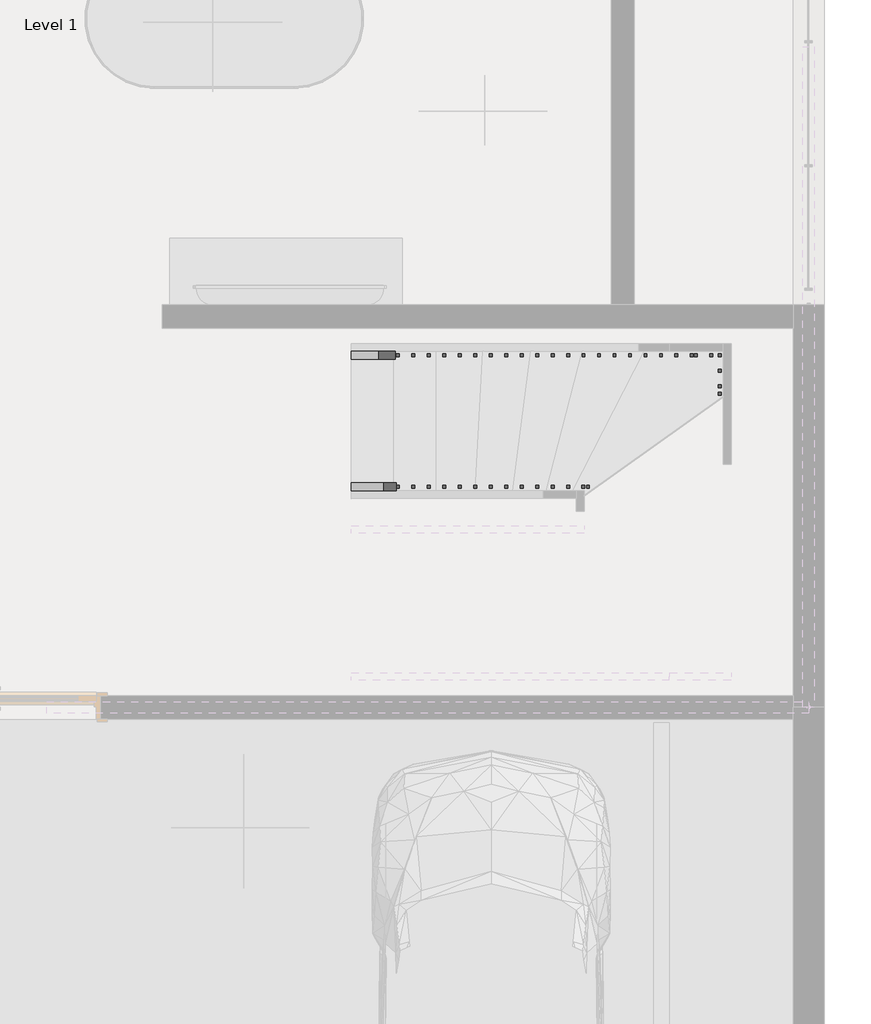
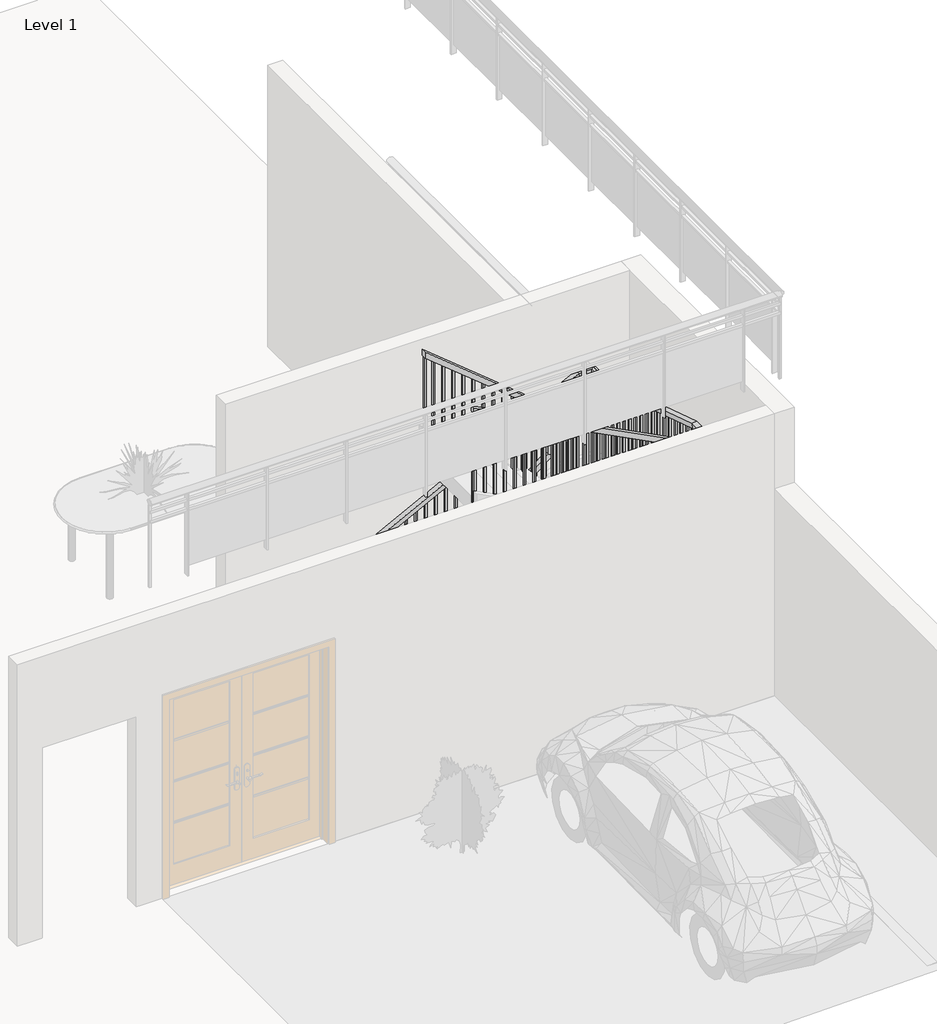
# One storey, part 4 of 6: 2 railings.
"""IFC4 building model written with IfcOpenShell, lengths in millimetres."""

from ifc_helpers import new_model, si_unit, frame, origin, place, context, project, spatial, polyline, outline, extrude, faceted_brep, element, save

model = new_model("IFC4")

# Units and contexts
model_context = context("Model", 3, world=origin())
ifc_project = project(units=[si_unit("LENGTHUNIT", "METRE", prefix="MILLI")], contexts=[model_context])

# Site, building, storey
site = spatial("IfcSite", under=ifc_project)
building = spatial("IfcBuilding", under=site)
storey = spatial("IfcBuildingStorey", under=building, Name="Level 1", Elevation=0.0)

# Railings
placement = place(None, origin())
element("IfcRailing", 1, ObjectType="Handrail - Rectangular", at=placement, inside=storey, context=model_context, shape_type="SolidModel", body=[
    faceted_brep([(-5314.5158104, 2829.6271763, 1025.2529681), (-5314.5158104, 2829.6271763, 959.7067088), (-5314.5158104, 2778.8271763, 959.7067088), (-5314.5158104, 2778.8271763, 1025.2529681), (-3862.9841185, 2829.6271763, 2208.7848338), (-3812.1841185, 2829.6271763, 2184.659247), (-3812.1841185, 2778.8271763, 2184.659247), (-3862.9841185, 2778.8271763, 2208.7848338), (-3862.9841185, 2829.6271763, 2414.6281882), (-3812.1841185, 2829.6271763, 2363.8281882), (-3812.1841185, 2778.8271763, 2363.8281882), (-3862.9841185, 2778.8271763, 2414.6281882), (-3735.9841185, 2829.6271763, 2414.6281882), (-3735.9841185, 2829.6271763, 2363.8281882), (-3786.7841185, 2778.8271763, 2363.8281882), (-3786.7841185, 2778.8271763, 2414.6281882), (-3735.9841185, 2702.6271763, 2414.6281882), (-3735.9841185, 2673.5058424, 2363.8281882), (-3786.7841185, 2673.5058424, 2363.8281882), (-3786.7841185, 2702.6271763, 2414.6281882), (-3735.9841185, 2575.6271763, 2631.5051451), (-3735.9841185, 2524.8271763, 2617.7256424), (-3786.7841185, 2524.8271763, 2617.7256424), (-3786.7841185, 2575.6271763, 2631.5051451), (-3735.9841185, 2575.6271763, 2837.3484995), (-3735.9841185, 2524.8271763, 2786.5484995), (-3786.7841185, 2524.8271763, 2786.5484995), (-3786.7841185, 2575.6271763, 2837.3484995), (-3735.9841185, 2448.6271763, 2837.3484995), (-3735.9841185, 2448.6271763, 2786.5484995), (-3786.7841185, 2499.4271763, 2786.5484995), (-3786.7841185, 2499.4271763, 2837.3484995), (-3862.9841185, 2448.6271763, 2837.3484995), (-3881.0695316, 2448.6271763, 2786.5484995), (-3881.0695316, 2499.4271763, 2786.5484995), (-3862.9841185, 2499.4271763, 2837.3484995), (-5314.5158104, 2448.6271763, 4020.8803652), (-5314.5158104, 2499.4271763, 4020.8803652), (-5314.5158104, 2499.4271763, 3955.3341059), (-5314.5158104, 2448.6271763, 3955.3341059)], [[[0, 1, 2, 3]], [[1, 0, 4, 5]], [[2, 1, 5, 6]], [[3, 2, 6, 7]], [[0, 3, 7, 4]], [[5, 4, 8, 9]], [[6, 5, 9, 10]], [[7, 6, 10, 11]], [[4, 7, 11, 8]], [[9, 8, 12, 13]], [[10, 9, 13, 14]], [[11, 10, 14, 15]], [[8, 11, 15, 12]], [[13, 12, 16, 17]], [[14, 13, 17, 18]], [[15, 14, 18, 19]], [[12, 15, 19, 16]], [[17, 16, 20, 21]], [[18, 17, 21, 22]], [[19, 18, 22, 23]], [[16, 19, 23, 20]], [[21, 20, 24, 25]], [[22, 21, 25, 26]], [[23, 22, 26, 27]], [[20, 23, 27, 24]], [[25, 24, 28, 29]], [[26, 25, 29, 30]], [[27, 26, 30, 31]], [[24, 27, 31, 28]], [[29, 28, 32, 33]], [[30, 29, 33, 34]], [[31, 30, 34, 35]], [[28, 31, 35, 32]], [[36, 37, 38, 39]], [[33, 32, 36, 39]], [[34, 33, 39, 38]], [[35, 34, 38, 37]], [[32, 35, 37, 36]]]),
    extrude(outline(polyline([(3866.2231262, -5205.2264749), (3881.7558784, -5224.2764749), (2878.6666667, -5224.2764749), (2878.6666667, -5205.2264749), (3866.2231262, -5205.2264749)])), frame((0.0, 2464.5021763, 0.0), z_axis=(0.0, 1.0, 0.0), x_axis=(0.0, 0.0, 1.0)), (0.0, 0.0, 1.0), 19.05),
    extrude(outline(polyline([(3783.3817813, -5103.6264749), (3798.9145334, -5122.6764749), (2878.6666667, -5122.6764749), (2878.6666667, -5103.6264749), (3783.3817813, -5103.6264749)])), frame((0.0, 2464.5021763, 0.0), z_axis=(0.0, 1.0, 0.0), x_axis=(0.0, 0.0, 1.0)), (0.0, 0.0, 1.0), 19.05),
    extrude(outline(polyline([(3700.5404364, -5002.0264749), (3716.0731885, -5021.0764749), (2709.3333333, -5021.0764749), (2709.3333333, -5002.0264749), (3700.5404364, -5002.0264749)])), frame((0.0, 2464.5021763, 0.0), z_axis=(0.0, 1.0, 0.0), x_axis=(0.0, 0.0, 1.0)), (0.0, 0.0, 1.0), 19.05),
    extrude(outline(polyline([(3617.6990914, -4900.4264749), (3633.2318436, -4919.4764749), (2709.3333333, -4919.4764749), (2709.3333333, -4900.4264749), (3617.6990914, -4900.4264749)])), frame((0.0, 2464.5021763, 0.0), z_axis=(0.0, 1.0, 0.0), x_axis=(0.0, 0.0, 1.0)), (0.0, 0.0, 1.0), 19.05),
    extrude(outline(polyline([(3534.8577465, -4798.8264749), (3550.3904987, -4817.8764749), (2709.3333333, -4817.8764749), (2709.3333333, -4798.8264749), (3534.8577465, -4798.8264749)])), frame((0.0, 2464.5021763, 0.0), z_axis=(0.0, 1.0, 0.0), x_axis=(0.0, 0.0, 1.0)), (0.0, 0.0, 1.0), 19.05),
    extrude(outline(polyline([(3452.0164016, -4697.2264749), (3467.5491538, -4716.2764749), (2540.0, -4716.2764749), (2540.0, -4697.2264749), (3452.0164016, -4697.2264749)])), frame((0.0, 2464.5021763, 0.0), z_axis=(0.0, 1.0, 0.0), x_axis=(0.0, 0.0, 1.0)), (0.0, 0.0, 1.0), 19.05),
    extrude(outline(polyline([(3369.1750567, -4595.6264749), (3384.7078088, -4614.6764749), (2540.0, -4614.6764749), (2540.0, -4595.6264749), (3369.1750567, -4595.6264749)])), frame((0.0, 2464.5021763, 0.0), z_axis=(0.0, 1.0, 0.0), x_axis=(0.0, 0.0, 1.0)), (0.0, 0.0, 1.0), 19.05),
    extrude(outline(polyline([(3286.3337117, -4494.0264749), (3301.8664639, -4513.0764749), (2540.0, -4513.0764749), (2540.0, -4494.0264749), (3286.3337117, -4494.0264749)])), frame((0.0, 2464.5021763, 0.0), z_axis=(0.0, 1.0, 0.0), x_axis=(0.0, 0.0, 1.0)), (0.0, 0.0, 1.0), 19.05),
    extrude(outline(polyline([(3203.4923668, -4392.4264749), (3219.025119, -4411.4764749), (2370.6666667, -4411.4764749), (2370.6666667, -4392.4264749), (3203.4923668, -4392.4264749)])), frame((0.0, 2464.5021763, 0.0), z_axis=(0.0, 1.0, 0.0), x_axis=(0.0, 0.0, 1.0)), (0.0, 0.0, 1.0), 19.05),
    extrude(outline(polyline([(3120.6510219, -4290.8264749), (3136.1837741, -4309.8764749), (2370.6666667, -4309.8764749), (2370.6666667, -4290.8264749), (3120.6510219, -4290.8264749)])), frame((0.0, 2464.5021763, 0.0), z_axis=(0.0, 1.0, 0.0), x_axis=(0.0, 0.0, 1.0)), (0.0, 0.0, 1.0), 19.05),
    extrude(outline(polyline([(3037.809677, -4189.2264749), (3053.3424291, -4208.2764749), (2201.3333333, -4208.2764749), (2201.3333333, -4189.2264749), (3037.809677, -4189.2264749)])), frame((0.0, 2464.5021763, 0.0), z_axis=(0.0, 1.0, 0.0), x_axis=(0.0, 0.0, 1.0)), (0.0, 0.0, 1.0), 19.05),
    extrude(outline(polyline([(2954.9683321, -4087.6264749), (2970.5010842, -4106.6764749), (2201.3333333, -4106.6764749), (2201.3333333, -4087.6264749), (2954.9683321, -4087.6264749)])), frame((0.0, 2464.5021763, 0.0), z_axis=(0.0, 1.0, 0.0), x_axis=(0.0, 0.0, 1.0)), (0.0, 0.0, 1.0), 19.05),
    extrude(outline(polyline([(2872.1269871, -3986.0264749), (2887.6597393, -4005.0764749), (2032.0, -4005.0764749), (2032.0, -3986.0264749), (2872.1269871, -3986.0264749)])), frame((0.0, 2464.5021763, 0.0), z_axis=(0.0, 1.0, 0.0), x_axis=(0.0, 0.0, 1.0)), (0.0, 0.0, 1.0), 19.05),
    extrude(outline(polyline([(2789.2856422, -3884.4264749), (2804.8183944, -3903.4764749), (2032.0, -3903.4764749), (2032.0, -3884.4264749), (2789.2856422, -3884.4264749)])), frame((0.0, 2464.5021763, 0.0), z_axis=(0.0, 1.0, 0.0), x_axis=(0.0, 0.0, 1.0)), (0.0, 0.0, 1.0), 19.05),
    extrude(outline(polyline([(2576.7162725, 2529.115018), (2595.7662725, 2496.5834745), (2595.7662725, 1524.0), (2576.7162725, 1524.0), (2576.7162725, 2529.115018)])), frame((-3770.9091185, 0.0, 0.0), z_axis=(1.0, 0.0, 0.0), x_axis=(0.0, 1.0, 0.0)), (0.0, 0.0, 1.0), 19.05),
    extrude(outline(polyline([(2678.3162725, 2355.6134525), (2697.3662725, 2323.0819089), (2697.3662725, 1524.0), (2678.3162725, 1524.0), (2678.3162725, 2355.6134525)])), frame((-3770.9091185, 0.0, 0.0), z_axis=(1.0, 0.0, 0.0), x_axis=(0.0, 1.0, 0.0)), (0.0, 0.0, 1.0), 19.05),
    extrude(outline(polyline([(2127.2519138, -3882.5908104), (2111.7191617, -3901.6408104), (1016.0, -3901.6408104), (1016.0, -3882.5908104), (2127.2519138, -3882.5908104)])), frame((0.0, 2794.7021763, 0.0), z_axis=(0.0, 1.0, 0.0), x_axis=(0.0, 0.0, 1.0)), (0.0, 0.0, 1.0), 19.05),
    extrude(outline(polyline([(2044.4105689, -3984.1908104), (2028.8778167, -4003.2408104), (1016.0, -4003.2408104), (1016.0, -3984.1908104), (2044.4105689, -3984.1908104)])), frame((0.0, 2794.7021763, 0.0), z_axis=(0.0, 1.0, 0.0), x_axis=(0.0, 0.0, 1.0)), (0.0, 0.0, 1.0), 19.05),
    extrude(outline(polyline([(1961.569224, -4085.7908104), (1946.0364718, -4104.8408104), (846.6666667, -4104.8408104), (846.6666667, -4085.7908104), (1961.569224, -4085.7908104)])), frame((0.0, 2794.7021763, 0.0), z_axis=(0.0, 1.0, 0.0), x_axis=(0.0, 0.0, 1.0)), (0.0, 0.0, 1.0), 19.05),
    extrude(outline(polyline([(1878.7278791, -4187.3908104), (1863.1951269, -4206.4408104), (846.6666667, -4206.4408104), (846.6666667, -4187.3908104), (1878.7278791, -4187.3908104)])), frame((0.0, 2794.7021763, 0.0), z_axis=(0.0, 1.0, 0.0), x_axis=(0.0, 0.0, 1.0)), (0.0, 0.0, 1.0), 19.05),
    extrude(outline(polyline([(1795.8865341, -4288.9908104), (1780.353782, -4308.0408104), (677.3333333, -4308.0408104), (677.3333333, -4288.9908104), (1795.8865341, -4288.9908104)])), frame((0.0, 2794.7021763, 0.0), z_axis=(0.0, 1.0, 0.0), x_axis=(0.0, 0.0, 1.0)), (0.0, 0.0, 1.0), 19.05),
    extrude(outline(polyline([(1713.0451892, -4390.5908104), (1697.5124371, -4409.6408104), (677.3333333, -4409.6408104), (677.3333333, -4390.5908104), (1713.0451892, -4390.5908104)])), frame((0.0, 2794.7021763, 0.0), z_axis=(0.0, 1.0, 0.0), x_axis=(0.0, 0.0, 1.0)), (0.0, 0.0, 1.0), 19.05),
    extrude(outline(polyline([(1630.2038443, -4492.1908104), (1614.6710921, -4511.2408104), (508.0, -4511.2408104), (508.0, -4492.1908104), (1630.2038443, -4492.1908104)])), frame((0.0, 2794.7021763, 0.0), z_axis=(0.0, 1.0, 0.0), x_axis=(0.0, 0.0, 1.0)), (0.0, 0.0, 1.0), 19.05),
    extrude(outline(polyline([(1547.3624994, -4593.7908104), (1531.8297472, -4612.8408104), (508.0, -4612.8408104), (508.0, -4593.7908104), (1547.3624994, -4593.7908104)])), frame((0.0, 2794.7021763, 0.0), z_axis=(0.0, 1.0, 0.0), x_axis=(0.0, 0.0, 1.0)), (0.0, 0.0, 1.0), 19.05),
    extrude(outline(polyline([(1464.5211545, -4695.3908104), (1448.9884023, -4714.4408104), (508.0, -4714.4408104), (508.0, -4695.3908104), (1464.5211545, -4695.3908104)])), frame((0.0, 2794.7021763, 0.0), z_axis=(0.0, 1.0, 0.0), x_axis=(0.0, 0.0, 1.0)), (0.0, 0.0, 1.0), 19.05),
    extrude(outline(polyline([(1381.6798095, -4796.9908104), (1366.1470574, -4816.0408104), (338.6666667, -4816.0408104), (338.6666667, -4796.9908104), (1381.6798095, -4796.9908104)])), frame((0.0, 2794.7021763, 0.0), z_axis=(0.0, 1.0, 0.0), x_axis=(0.0, 0.0, 1.0)), (0.0, 0.0, 1.0), 19.05),
    extrude(outline(polyline([(1298.8384646, -4898.5908104), (1283.3057124, -4917.6408104), (338.6666667, -4917.6408104), (338.6666667, -4898.5908104), (1298.8384646, -4898.5908104)])), frame((0.0, 2794.7021763, 0.0), z_axis=(0.0, 1.0, 0.0), x_axis=(0.0, 0.0, 1.0)), (0.0, 0.0, 1.0), 19.05),
    extrude(outline(polyline([(1215.9971197, -5000.1908104), (1200.4643675, -5019.2408104), (338.6666667, -5019.2408104), (338.6666667, -5000.1908104), (1215.9971197, -5000.1908104)])), frame((0.0, 2794.7021763, 0.0), z_axis=(0.0, 1.0, 0.0), x_axis=(0.0, 0.0, 1.0)), (0.0, 0.0, 1.0), 19.05),
    extrude(outline(polyline([(1133.1557748, -5101.7908104), (1117.6230226, -5120.8408104), (169.3333333, -5120.8408104), (169.3333333, -5101.7908104), (1133.1557748, -5101.7908104)])), frame((0.0, 2794.7021763, 0.0), z_axis=(0.0, 1.0, 0.0), x_axis=(0.0, 0.0, 1.0)), (0.0, 0.0, 1.0), 19.05),
    extrude(outline(polyline([(1050.3144298, -5203.3908104), (1034.7816777, -5222.4408104), (169.3333333, -5222.4408104), (169.3333333, -5203.3908104), (1050.3144298, -5203.3908104)])), frame((0.0, 2794.7021763, 0.0), z_axis=(0.0, 1.0, 0.0), x_axis=(0.0, 0.0, 1.0)), (0.0, 0.0, 1.0), 19.05),
    extrude(outline(polyline([(-3782.8264749, 2483.5521763), (-3782.8264749, 2464.5021763), (-3801.8764749, 2464.5021763), (-3801.8764749, 2483.5521763), (-3782.8264749, 2483.5521763)])), frame((0.0, 0.0, 1862.6666667), z_axis=(0.0, 0.0, 1.0), x_axis=(1.0, 0.0, 0.0)), (0.0, 0.0, 1.0), 923.8818329),
    extrude(outline(polyline([(-3770.9091185, 2483.5521763), (-3751.8591185, 2483.5521763), (-3751.8591185, 2464.5021763), (-3770.9091185, 2464.5021763), (-3770.9091185, 2483.5521763)])), frame((0.0, 0.0, 1862.6666667), z_axis=(0.0, 0.0, 1.0), x_axis=(1.0, 0.0, 0.0)), (0.0, 0.0, 1.0), 923.8818329),
    extrude(outline(polyline([(-3770.9091185, 2498.33808), (-3751.8591185, 2498.33808), (-3751.8591185, 2479.28808), (-3770.9091185, 2479.28808), (-3770.9091185, 2498.33808)])), frame((0.0, 0.0, 1693.3333333), z_axis=(0.0, 0.0, 1.0), x_axis=(1.0, 0.0, 0.0)), (0.0, 0.0, 1.0), 1093.2151662),
    extrude(outline(polyline([(-3770.9091185, 2798.9662725), (-3751.8591185, 2798.9662725), (-3751.8591185, 2779.9162725), (-3770.9091185, 2779.9162725), (-3770.9091185, 2798.9662725)])), frame((0.0, 0.0, 1354.6666667), z_axis=(0.0, 0.0, 1.0), x_axis=(1.0, 0.0, 0.0)), (0.0, 0.0, 1.0), 1009.1615215),
    extrude(outline(polyline([(-3770.9091185, 2794.7021763), (-3770.9091185, 2813.7521763), (-3751.8591185, 2813.7521763), (-3751.8591185, 2794.7021763), (-3770.9091185, 2794.7021763)])), frame((0.0, 0.0, 1185.3333333), z_axis=(0.0, 0.0, 1.0), x_axis=(1.0, 0.0, 0.0)), (0.0, 0.0, 1.0), 1178.4948549),
    extrude(outline(polyline([(-3801.8764749, 2794.7021763), (-3801.8764749, 2813.7521763), (-3782.8264749, 2813.7521763), (-3782.8264749, 2794.7021763), (-3801.8764749, 2794.7021763)])), frame((0.0, 0.0, 1185.3333333), z_axis=(0.0, 0.0, 1.0), x_axis=(1.0, 0.0, 0.0)), (0.0, 0.0, 1.0), 1178.4948549),
    extrude(outline(polyline([(3939.8013537, -5295.4658104), (3955.3341059, -5314.5158104), (2878.6666667, -5314.5158104), (2878.6666667, -5295.4658104), (3939.8013537, -5295.4658104)])), frame((0.0, 2464.5021763, 0.0), z_axis=(0.0, 1.0, 0.0), x_axis=(0.0, 0.0, 1.0)), (0.0, 0.0, 1.0), 19.05),
    extrude(outline(polyline([(975.239461, -5295.4658104), (959.7067088, -5314.5158104), (169.3333333, -5314.5158104), (169.3333333, -5295.4658104), (975.239461, -5295.4658104)])), frame((0.0, 2794.7021763, 0.0), z_axis=(0.0, 1.0, 0.0), x_axis=(0.0, 0.0, 1.0)), (0.0, 0.0, 1.0), 19.05),
])
element("IfcRailing", 2, ObjectType="Handrail - Rectangular", at=placement, inside=storey, context=model_context, shape_type="SolidModel", body=[
    faceted_brep([(-5314.5158104, 3693.2271763, 1109.0771751), (-5314.5158104, 3693.2271763, 1051.9280057), (-5314.5158104, 3642.4271763, 1051.9280057), (-5314.5158104, 3642.4271763, 1109.0771751), (-3054.5339539, 3693.2271763, 2273.7644996), (-3042.2139026, 3693.2271763, 2222.9644996), (-3042.2139026, 3642.4271763, 2222.9644996), (-3054.5339539, 3642.4271763, 2273.7644996), (-2872.3841185, 3693.2271763, 2273.7644996), (-2872.3841185, 3693.2271763, 2222.9644996), (-2923.1841185, 3642.4271763, 2222.9644996), (-2923.1841185, 3642.4271763, 2273.7644996), (-2872.3841185, 3416.0732236, 2273.7644996), (-2872.3841185, 3408.1226475, 2222.9644996), (-2923.1841185, 3408.1226475, 2222.9644996), (-2923.1841185, 3416.0732236, 2273.7644996), (-2872.3841185, 1862.1811289, 2772.3688337), (-2872.3841185, 1854.2305527, 2721.5688337), (-2923.1841185, 1854.2305527, 2721.5688337), (-2923.1841185, 1862.1811289, 2772.3688337), (-2872.3841185, 1585.0271763, 2772.3688337), (-2872.3841185, 1585.0271763, 2721.5688337), (-2923.1841185, 1635.8271763, 2721.5688337), (-2923.1841185, 1635.8271763, 2772.3688337), (-3054.5339539, 1585.0271763, 2772.3688337), (-3066.8540052, 1585.0271763, 2721.5688337), (-3066.8540052, 1635.8271763, 2721.5688337), (-3054.5339539, 1635.8271763, 2772.3688337), (-5314.5158104, 1585.0271763, 3937.0561582), (-5314.5158104, 1635.8271763, 3937.0561582), (-5314.5158104, 1635.8271763, 3879.9069889), (-5314.5158104, 1585.0271763, 3879.9069889)], [[[0, 1, 2, 3]], [[1, 0, 4, 5]], [[2, 1, 5, 6]], [[3, 2, 6, 7]], [[0, 3, 7, 4]], [[5, 4, 8, 9]], [[6, 5, 9, 10]], [[7, 6, 10, 11]], [[4, 7, 11, 8]], [[9, 8, 12, 13]], [[10, 9, 13, 14]], [[11, 10, 14, 15]], [[8, 11, 15, 12]], [[13, 12, 16, 17]], [[14, 13, 17, 18]], [[15, 14, 18, 19]], [[12, 15, 19, 16]], [[17, 16, 20, 21]], [[18, 17, 21, 22]], [[19, 18, 22, 23]], [[16, 19, 23, 20]], [[21, 20, 24, 25]], [[22, 21, 25, 26]], [[23, 22, 26, 27]], [[20, 23, 27, 24]], [[28, 29, 30, 31]], [[25, 24, 28, 31]], [[26, 25, 31, 30]], [[27, 26, 30, 29]], [[24, 27, 29, 28]]]),
    extrude(outline(polyline([(3872.0443296, -5299.2589539), (2878.6666667, -5299.2589539), (2878.6666667, -5280.2089539), (3862.2268642, -5280.2089539), (3872.0443296, -5299.2589539)])), frame((0.0, 1600.9021763, 0.0), z_axis=(0.0, 1.0, 0.0), x_axis=(0.0, 0.0, 1.0)), (0.0, 0.0, 1.0), 19.05),
    extrude(outline(polyline([(3819.6845145, -5197.6589539), (2878.6666667, -5197.6589539), (2878.6666667, -5178.6089539), (3809.8670491, -5178.6089539), (3819.6845145, -5197.6589539)])), frame((0.0, 1600.9021763, 0.0), z_axis=(0.0, 1.0, 0.0), x_axis=(0.0, 0.0, 1.0)), (0.0, 0.0, 1.0), 19.05),
    extrude(outline(polyline([(3767.3246993, -5096.0589539), (2878.6666667, -5096.0589539), (2878.6666667, -5077.0089539), (3757.507234, -5077.0089539), (3767.3246993, -5096.0589539)])), frame((0.0, 1600.9021763, 0.0), z_axis=(0.0, 1.0, 0.0), x_axis=(0.0, 0.0, 1.0)), (0.0, 0.0, 1.0), 19.05),
    extrude(outline(polyline([(3714.9648842, -4994.4589539), (2709.3333333, -4994.4589539), (2709.3333333, -4975.4089539), (3705.1474189, -4975.4089539), (3714.9648842, -4994.4589539)])), frame((0.0, 1600.9021763, 0.0), z_axis=(0.0, 1.0, 0.0), x_axis=(0.0, 0.0, 1.0)), (0.0, 0.0, 1.0), 19.05),
    extrude(outline(polyline([(3662.6050691, -4892.8589539), (2709.3333333, -4892.8589539), (2709.3333333, -4873.8089539), (3652.7876038, -4873.8089539), (3662.6050691, -4892.8589539)])), frame((0.0, 1600.9021763, 0.0), z_axis=(0.0, 1.0, 0.0), x_axis=(0.0, 0.0, 1.0)), (0.0, 0.0, 1.0), 19.05),
    extrude(outline(polyline([(3610.245254, -4791.2589539), (2709.3333333, -4791.2589539), (2709.3333333, -4772.2089539), (3600.4277887, -4772.2089539), (3610.245254, -4791.2589539)])), frame((0.0, 1600.9021763, 0.0), z_axis=(0.0, 1.0, 0.0), x_axis=(0.0, 0.0, 1.0)), (0.0, 0.0, 1.0), 19.05),
    extrude(outline(polyline([(3557.8854389, -4689.6589539), (2540.0, -4689.6589539), (2540.0, -4670.6089539), (3548.0679735, -4670.6089539), (3557.8854389, -4689.6589539)])), frame((0.0, 1600.9021763, 0.0), z_axis=(0.0, 1.0, 0.0), x_axis=(0.0, 0.0, 1.0)), (0.0, 0.0, 1.0), 19.05),
    extrude(outline(polyline([(3505.5256238, -4588.0589539), (2540.0, -4588.0589539), (2540.0, -4569.0089539), (3495.7081584, -4569.0089539), (3505.5256238, -4588.0589539)])), frame((0.0, 1600.9021763, 0.0), z_axis=(0.0, 1.0, 0.0), x_axis=(0.0, 0.0, 1.0)), (0.0, 0.0, 1.0), 19.05),
    extrude(outline(polyline([(3453.1658086, -4486.4589539), (2540.0, -4486.4589539), (2540.0, -4467.4089539), (3443.3483433, -4467.4089539), (3453.1658086, -4486.4589539)])), frame((0.0, 1600.9021763, 0.0), z_axis=(0.0, 1.0, 0.0), x_axis=(0.0, 0.0, 1.0)), (0.0, 0.0, 1.0), 19.05),
    extrude(outline(polyline([(3400.8059935, -4384.8589539), (2370.6666667, -4384.8589539), (2370.6666667, -4365.8089539), (3390.9885282, -4365.8089539), (3400.8059935, -4384.8589539)])), frame((0.0, 1600.9021763, 0.0), z_axis=(0.0, 1.0, 0.0), x_axis=(0.0, 0.0, 1.0)), (0.0, 0.0, 1.0), 19.05),
    extrude(outline(polyline([(3348.4461784, -4283.2589539), (2370.6666667, -4283.2589539), (2370.6666667, -4264.2089539), (3338.6287131, -4264.2089539), (3348.4461784, -4283.2589539)])), frame((0.0, 1600.9021763, 0.0), z_axis=(0.0, 1.0, 0.0), x_axis=(0.0, 0.0, 1.0)), (0.0, 0.0, 1.0), 19.05),
    extrude(outline(polyline([(3296.0863633, -4181.6589539), (2370.6666667, -4181.6589539), (2370.6666667, -4162.6089539), (3286.268898, -4162.6089539), (3296.0863633, -4181.6589539)])), frame((0.0, 1600.9021763, 0.0), z_axis=(0.0, 1.0, 0.0), x_axis=(0.0, 0.0, 1.0)), (0.0, 0.0, 1.0), 19.05),
    extrude(outline(polyline([(3243.7265482, -4080.0589539), (2201.3333333, -4080.0589539), (2201.3333333, -4061.0089539), (3233.9090828, -4061.0089539), (3243.7265482, -4080.0589539)])), frame((0.0, 1600.9021763, 0.0), z_axis=(0.0, 1.0, 0.0), x_axis=(0.0, 0.0, 1.0)), (0.0, 0.0, 1.0), 19.05),
    extrude(outline(polyline([(3191.3667331, -3978.4589539), (2201.3333333, -3978.4589539), (2201.3333333, -3959.4089539), (3181.5492677, -3959.4089539), (3191.3667331, -3978.4589539)])), frame((0.0, 1600.9021763, 0.0), z_axis=(0.0, 1.0, 0.0), x_axis=(0.0, 0.0, 1.0)), (0.0, 0.0, 1.0), 19.05),
    extrude(outline(polyline([(3139.0069179, -3876.8589539), (2201.3333333, -3876.8589539), (2201.3333333, -3857.8089539), (3129.1894526, -3857.8089539), (3139.0069179, -3876.8589539)])), frame((0.0, 1600.9021763, 0.0), z_axis=(0.0, 1.0, 0.0), x_axis=(0.0, 0.0, 1.0)), (0.0, 0.0, 1.0), 19.05),
    extrude(outline(polyline([(3086.6471028, -3775.2589539), (2032.0, -3775.2589539), (2032.0, -3756.2089539), (3076.8296375, -3756.2089539), (3086.6471028, -3775.2589539)])), frame((0.0, 1600.9021763, 0.0), z_axis=(0.0, 1.0, 0.0), x_axis=(0.0, 0.0, 1.0)), (0.0, 0.0, 1.0), 19.05),
    extrude(outline(polyline([(3034.2872877, -3673.6589539), (2032.0, -3673.6589539), (2032.0, -3654.6089539), (3024.4698224, -3654.6089539), (3034.2872877, -3673.6589539)])), frame((0.0, 1600.9021763, 0.0), z_axis=(0.0, 1.0, 0.0), x_axis=(0.0, 0.0, 1.0)), (0.0, 0.0, 1.0), 19.05),
    extrude(outline(polyline([(2981.9274726, -3572.0589539), (2032.0, -3572.0589539), (2032.0, -3553.0089539), (2972.1100073, -3553.0089539), (2981.9274726, -3572.0589539)])), frame((0.0, 1600.9021763, 0.0), z_axis=(0.0, 1.0, 0.0), x_axis=(0.0, 0.0, 1.0)), (0.0, 0.0, 1.0), 19.05),
    extrude(outline(polyline([(2929.5676575, -3470.4589539), (2032.0, -3470.4589539), (2032.0, -3451.4089539), (2919.7501921, -3451.4089539), (2929.5676575, -3470.4589539)])), frame((0.0, 1600.9021763, 0.0), z_axis=(0.0, 1.0, 0.0), x_axis=(0.0, 0.0, 1.0)), (0.0, 0.0, 1.0), 19.05),
    extrude(outline(polyline([(2877.2078424, -3368.8589539), (1862.6666667, -3368.8589539), (1862.6666667, -3349.8089539), (2867.390377, -3349.8089539), (2877.2078424, -3368.8589539)])), frame((0.0, 1600.9021763, 0.0), z_axis=(0.0, 1.0, 0.0), x_axis=(0.0, 0.0, 1.0)), (0.0, 0.0, 1.0), 19.05),
    extrude(outline(polyline([(2824.8480272, -3267.2589539), (1862.6666667, -3267.2589539), (1862.6666667, -3248.2089539), (2815.0305619, -3248.2089539), (2824.8480272, -3267.2589539)])), frame((0.0, 1600.9021763, 0.0), z_axis=(0.0, 1.0, 0.0), x_axis=(0.0, 0.0, 1.0)), (0.0, 0.0, 1.0), 19.05),
    extrude(outline(polyline([(2772.4882121, -3165.6589539), (1862.6666667, -3165.6589539), (1862.6666667, -3146.6089539), (2762.6707468, -3146.6089539), (2772.4882121, -3165.6589539)])), frame((0.0, 1600.9021763, 0.0), z_axis=(0.0, 1.0, 0.0), x_axis=(0.0, 0.0, 1.0)), (0.0, 0.0, 1.0), 19.05),
    extrude(outline(polyline([(-2989.8591185, 1600.9021763), (-3008.9091185, 1600.9021763), (-3008.9091185, 1619.9521763), (-2989.8591185, 1619.9521763), (-2989.8591185, 1600.9021763)])), frame((0.0, 0.0, 1862.6666667), z_axis=(0.0, 0.0, 1.0), x_axis=(1.0, 0.0, 0.0)), (0.0, 0.0, 1.0), 858.902167),
    extrude(outline(polyline([(-2888.2591185, 1668.5061289), (-2888.2591185, 1649.4561289), (-2907.3091185, 1649.4561289), (-2907.3091185, 1668.5061289), (-2888.2591185, 1668.5061289)])), frame((0.0, 0.0, 1862.6666667), z_axis=(0.0, 0.0, 1.0), x_axis=(1.0, 0.0, 0.0)), (0.0, 0.0, 1.0), 858.902167),
    extrude(outline(polyline([(-2888.2591185, 1770.1061289), (-2888.2591185, 1751.0561289), (-2907.3091185, 1751.0561289), (-2907.3091185, 1770.1061289), (-2888.2591185, 1770.1061289)])), frame((0.0, 0.0, 1862.6666667), z_axis=(0.0, 0.0, 1.0), x_axis=(1.0, 0.0, 0.0)), (0.0, 0.0, 1.0), 858.902167),
    extrude(outline(polyline([(1901.5982236, 2706.3697564), (1901.5982236, 1693.3333333), (1882.5482236, 1693.3333333), (1882.5482236, 2712.4824155), (1901.5982236, 2706.3697564)])), frame((-2907.3091185, 0.0, 0.0), z_axis=(1.0, 0.0, 0.0), x_axis=(0.0, 1.0, 0.0)), (0.0, 0.0, 1.0), 19.05),
    extrude(outline(polyline([(2003.1982236, 2673.7689082), (2003.1982236, 1693.3333333), (1984.1482236, 1693.3333333), (1984.1482236, 2679.8815673), (2003.1982236, 2673.7689082)])), frame((-2907.3091185, 0.0, 0.0), z_axis=(1.0, 0.0, 0.0), x_axis=(0.0, 1.0, 0.0)), (0.0, 0.0, 1.0), 19.05),
    extrude(outline(polyline([(2104.7982236, 2641.16806), (2104.7982236, 1693.3333333), (2085.7482236, 1693.3333333), (2085.7482236, 2647.280719), (2104.7982236, 2641.16806)])), frame((-2907.3091185, 0.0, 0.0), z_axis=(1.0, 0.0, 0.0), x_axis=(0.0, 1.0, 0.0)), (0.0, 0.0, 1.0), 19.05),
    extrude(outline(polyline([(2206.3982236, 2608.5672118), (2206.3982236, 1693.3333333), (2187.3482236, 1693.3333333), (2187.3482236, 2614.6798708), (2206.3982236, 2608.5672118)])), frame((-2907.3091185, 0.0, 0.0), z_axis=(1.0, 0.0, 0.0), x_axis=(0.0, 1.0, 0.0)), (0.0, 0.0, 1.0), 19.05),
    extrude(outline(polyline([(2307.9982236, 2575.9663635), (2307.9982236, 1693.3333333), (2288.9482236, 1693.3333333), (2288.9482236, 2582.0790226), (2307.9982236, 2575.9663635)])), frame((-2907.3091185, 0.0, 0.0), z_axis=(1.0, 0.0, 0.0), x_axis=(0.0, 1.0, 0.0)), (0.0, 0.0, 1.0), 19.05),
    extrude(outline(polyline([(2409.5982236, 2543.3655153), (2409.5982236, 1693.3333333), (2390.5482236, 1693.3333333), (2390.5482236, 2549.4781744), (2409.5982236, 2543.3655153)])), frame((-2907.3091185, 0.0, 0.0), z_axis=(1.0, 0.0, 0.0), x_axis=(0.0, 1.0, 0.0)), (0.0, 0.0, 1.0), 19.05),
    extrude(outline(polyline([(2511.1982236, 2510.7646671), (2511.1982236, 1524.0), (2492.1482236, 1524.0), (2492.1482236, 2516.8773261), (2511.1982236, 2510.7646671)])), frame((-2907.3091185, 0.0, 0.0), z_axis=(1.0, 0.0, 0.0), x_axis=(0.0, 1.0, 0.0)), (0.0, 0.0, 1.0), 19.05),
    extrude(outline(polyline([(2612.7982236, 2478.1638189), (2612.7982236, 1524.0), (2593.7482236, 1524.0), (2593.7482236, 2484.2764779), (2612.7982236, 2478.1638189)])), frame((-2907.3091185, 0.0, 0.0), z_axis=(1.0, 0.0, 0.0), x_axis=(0.0, 1.0, 0.0)), (0.0, 0.0, 1.0), 19.05),
    extrude(outline(polyline([(2714.3982236, 2445.5629706), (2714.3982236, 1524.0), (2695.3482236, 1524.0), (2695.3482236, 2451.6756297), (2714.3982236, 2445.5629706)])), frame((-2907.3091185, 0.0, 0.0), z_axis=(1.0, 0.0, 0.0), x_axis=(0.0, 1.0, 0.0)), (0.0, 0.0, 1.0), 19.05),
    extrude(outline(polyline([(2815.9982236, 2412.9621224), (2815.9982236, 1524.0), (2796.9482236, 1524.0), (2796.9482236, 2419.0747814), (2815.9982236, 2412.9621224)])), frame((-2907.3091185, 0.0, 0.0), z_axis=(1.0, 0.0, 0.0), x_axis=(0.0, 1.0, 0.0)), (0.0, 0.0, 1.0), 19.05),
    extrude(outline(polyline([(2917.5982236, 2380.3612742), (2917.5982236, 1354.6666667), (2898.5482236, 1354.6666667), (2898.5482236, 2386.4739332), (2917.5982236, 2380.3612742)])), frame((-2907.3091185, 0.0, 0.0), z_axis=(1.0, 0.0, 0.0), x_axis=(0.0, 1.0, 0.0)), (0.0, 0.0, 1.0), 19.05),
    extrude(outline(polyline([(3019.1982236, 2347.7604259), (3019.1982236, 1354.6666667), (3000.1482236, 1354.6666667), (3000.1482236, 2353.873085), (3019.1982236, 2347.7604259)])), frame((-2907.3091185, 0.0, 0.0), z_axis=(1.0, 0.0, 0.0), x_axis=(0.0, 1.0, 0.0)), (0.0, 0.0, 1.0), 19.05),
    extrude(outline(polyline([(3120.7982236, 2315.1595777), (3120.7982236, 1354.6666667), (3101.7482236, 1354.6666667), (3101.7482236, 2321.2722368), (3120.7982236, 2315.1595777)])), frame((-2907.3091185, 0.0, 0.0), z_axis=(1.0, 0.0, 0.0), x_axis=(0.0, 1.0, 0.0)), (0.0, 0.0, 1.0), 19.05),
    extrude(outline(polyline([(3222.3982236, 2282.5587295), (3222.3982236, 1354.6666667), (3203.3482236, 1354.6666667), (3203.3482236, 2288.6713885), (3222.3982236, 2282.5587295)])), frame((-2907.3091185, 0.0, 0.0), z_axis=(1.0, 0.0, 0.0), x_axis=(0.0, 1.0, 0.0)), (0.0, 0.0, 1.0), 19.05),
    extrude(outline(polyline([(3323.9982236, 2249.9578813), (3323.9982236, 1354.6666667), (3304.9482236, 1354.6666667), (3304.9482236, 2256.0705403), (3323.9982236, 2249.9578813)])), frame((-2907.3091185, 0.0, 0.0), z_axis=(1.0, 0.0, 0.0), x_axis=(0.0, 1.0, 0.0)), (0.0, 0.0, 1.0), 19.05),
    extrude(outline(polyline([(-2888.2591185, 3474.1521763), (-2888.2591185, 3455.1021763), (-2907.3091185, 3455.1021763), (-2907.3091185, 3474.1521763), (-2888.2591185, 3474.1521763)])), frame((0.0, 0.0, 1185.3333333), z_axis=(0.0, 0.0, 1.0), x_axis=(1.0, 0.0, 0.0)), (0.0, 0.0, 1.0), 1037.6311663),
    extrude(outline(polyline([(-2888.2591185, 3575.7521763), (-2888.2591185, 3556.7021763), (-2907.3091185, 3556.7021763), (-2907.3091185, 3575.7521763), (-2888.2591185, 3575.7521763)])), frame((0.0, 0.0, 1185.3333333), z_axis=(0.0, 0.0, 1.0), x_axis=(1.0, 0.0, 0.0)), (0.0, 0.0, 1.0), 1037.6311663),
    extrude(outline(polyline([(-2962.4589539, 3677.3521763), (-2943.4089539, 3677.3521763), (-2943.4089539, 3658.3021763), (-2962.4589539, 3658.3021763), (-2962.4589539, 3677.3521763)])), frame((0.0, 0.0, 1185.3333333), z_axis=(0.0, 0.0, 1.0), x_axis=(1.0, 0.0, 0.0)), (0.0, 0.0, 1.0), 1037.6311663),
    extrude(outline(polyline([(2198.9352056, -3088.8408104), (1185.3333333, -3088.8408104), (1185.3333333, -3069.7908104), (2208.752671, -3069.7908104), (2198.9352056, -3088.8408104)])), frame((0.0, 3658.3021763, 0.0), z_axis=(0.0, 1.0, 0.0), x_axis=(0.0, 0.0, 1.0)), (0.0, 0.0, 1.0), 19.05),
    extrude(outline(polyline([(2146.5753905, -3190.4408104), (1185.3333333, -3190.4408104), (1185.3333333, -3171.3908104), (2156.3928558, -3171.3908104), (2146.5753905, -3190.4408104)])), frame((0.0, 3658.3021763, 0.0), z_axis=(0.0, 1.0, 0.0), x_axis=(0.0, 0.0, 1.0)), (0.0, 0.0, 1.0), 19.05),
    extrude(outline(polyline([(2094.2155754, -3292.0408104), (1185.3333333, -3292.0408104), (1185.3333333, -3272.9908104), (2104.0330407, -3272.9908104), (2094.2155754, -3292.0408104)])), frame((0.0, 3658.3021763, 0.0), z_axis=(0.0, 1.0, 0.0), x_axis=(0.0, 0.0, 1.0)), (0.0, 0.0, 1.0), 19.05),
    extrude(outline(polyline([(2041.8557603, -3393.6408104), (1185.3333333, -3393.6408104), (1185.3333333, -3374.5908104), (2051.6732256, -3374.5908104), (2041.8557603, -3393.6408104)])), frame((0.0, 3658.3021763, 0.0), z_axis=(0.0, 1.0, 0.0), x_axis=(0.0, 0.0, 1.0)), (0.0, 0.0, 1.0), 19.05),
    extrude(outline(polyline([(1989.4959452, -3495.2408104), (1016.0, -3495.2408104), (1016.0, -3476.1908104), (1999.3134105, -3476.1908104), (1989.4959452, -3495.2408104)])), frame((0.0, 3658.3021763, 0.0), z_axis=(0.0, 1.0, 0.0), x_axis=(0.0, 0.0, 1.0)), (0.0, 0.0, 1.0), 19.05),
    extrude(outline(polyline([(1937.13613, -3596.8408104), (1016.0, -3596.8408104), (1016.0, -3577.7908104), (1946.9535954, -3577.7908104), (1937.13613, -3596.8408104)])), frame((0.0, 3658.3021763, 0.0), z_axis=(0.0, 1.0, 0.0), x_axis=(0.0, 0.0, 1.0)), (0.0, 0.0, 1.0), 19.05),
    extrude(outline(polyline([(1884.7763149, -3698.4408104), (1016.0, -3698.4408104), (1016.0, -3679.3908104), (1894.5937803, -3679.3908104), (1884.7763149, -3698.4408104)])), frame((0.0, 3658.3021763, 0.0), z_axis=(0.0, 1.0, 0.0), x_axis=(0.0, 0.0, 1.0)), (0.0, 0.0, 1.0), 19.05),
    extrude(outline(polyline([(1832.4164998, -3800.0408104), (1016.0, -3800.0408104), (1016.0, -3780.9908104), (1842.2339651, -3780.9908104), (1832.4164998, -3800.0408104)])), frame((0.0, 3658.3021763, 0.0), z_axis=(0.0, 1.0, 0.0), x_axis=(0.0, 0.0, 1.0)), (0.0, 0.0, 1.0), 19.05),
    extrude(outline(polyline([(1780.0566847, -3901.6408104), (846.6666667, -3901.6408104), (846.6666667, -3882.5908104), (1789.87415, -3882.5908104), (1780.0566847, -3901.6408104)])), frame((0.0, 3658.3021763, 0.0), z_axis=(0.0, 1.0, 0.0), x_axis=(0.0, 0.0, 1.0)), (0.0, 0.0, 1.0), 19.05),
    extrude(outline(polyline([(1727.6968696, -4003.2408104), (846.6666667, -4003.2408104), (846.6666667, -3984.1908104), (1737.5143349, -3984.1908104), (1727.6968696, -4003.2408104)])), frame((0.0, 3658.3021763, 0.0), z_axis=(0.0, 1.0, 0.0), x_axis=(0.0, 0.0, 1.0)), (0.0, 0.0, 1.0), 19.05),
    extrude(outline(polyline([(1675.3370545, -4104.8408104), (846.6666667, -4104.8408104), (846.6666667, -4085.7908104), (1685.1545198, -4085.7908104), (1675.3370545, -4104.8408104)])), frame((0.0, 3658.3021763, 0.0), z_axis=(0.0, 1.0, 0.0), x_axis=(0.0, 0.0, 1.0)), (0.0, 0.0, 1.0), 19.05),
    extrude(outline(polyline([(1622.9772393, -4206.4408104), (677.3333333, -4206.4408104), (677.3333333, -4187.3908104), (1632.7947047, -4187.3908104), (1622.9772393, -4206.4408104)])), frame((0.0, 3658.3021763, 0.0), z_axis=(0.0, 1.0, 0.0), x_axis=(0.0, 0.0, 1.0)), (0.0, 0.0, 1.0), 19.05),
    extrude(outline(polyline([(1570.6174242, -4308.0408104), (677.3333333, -4308.0408104), (677.3333333, -4288.9908104), (1580.4348896, -4288.9908104), (1570.6174242, -4308.0408104)])), frame((0.0, 3658.3021763, 0.0), z_axis=(0.0, 1.0, 0.0), x_axis=(0.0, 0.0, 1.0)), (0.0, 0.0, 1.0), 19.05),
    extrude(outline(polyline([(1518.2576091, -4409.6408104), (677.3333333, -4409.6408104), (677.3333333, -4390.5908104), (1528.0750744, -4390.5908104), (1518.2576091, -4409.6408104)])), frame((0.0, 3658.3021763, 0.0), z_axis=(0.0, 1.0, 0.0), x_axis=(0.0, 0.0, 1.0)), (0.0, 0.0, 1.0), 19.05),
    extrude(outline(polyline([(1465.897794, -4511.2408104), (508.0, -4511.2408104), (508.0, -4492.1908104), (1475.7152593, -4492.1908104), (1465.897794, -4511.2408104)])), frame((0.0, 3658.3021763, 0.0), z_axis=(0.0, 1.0, 0.0), x_axis=(0.0, 0.0, 1.0)), (0.0, 0.0, 1.0), 19.05),
    extrude(outline(polyline([(1413.5379789, -4612.8408104), (508.0, -4612.8408104), (508.0, -4593.7908104), (1423.3554442, -4593.7908104), (1413.5379789, -4612.8408104)])), frame((0.0, 3658.3021763, 0.0), z_axis=(0.0, 1.0, 0.0), x_axis=(0.0, 0.0, 1.0)), (0.0, 0.0, 1.0), 19.05),
    extrude(outline(polyline([(1361.1781638, -4714.4408104), (508.0, -4714.4408104), (508.0, -4695.3908104), (1370.9956291, -4695.3908104), (1361.1781638, -4714.4408104)])), frame((0.0, 3658.3021763, 0.0), z_axis=(0.0, 1.0, 0.0), x_axis=(0.0, 0.0, 1.0)), (0.0, 0.0, 1.0), 19.05),
    extrude(outline(polyline([(1308.8183486, -4816.0408104), (338.6666667, -4816.0408104), (338.6666667, -4796.9908104), (1318.635814, -4796.9908104), (1308.8183486, -4816.0408104)])), frame((0.0, 3658.3021763, 0.0), z_axis=(0.0, 1.0, 0.0), x_axis=(0.0, 0.0, 1.0)), (0.0, 0.0, 1.0), 19.05),
    extrude(outline(polyline([(1256.4585335, -4917.6408104), (338.6666667, -4917.6408104), (338.6666667, -4898.5908104), (1266.2759989, -4898.5908104), (1256.4585335, -4917.6408104)])), frame((0.0, 3658.3021763, 0.0), z_axis=(0.0, 1.0, 0.0), x_axis=(0.0, 0.0, 1.0)), (0.0, 0.0, 1.0), 19.05),
    extrude(outline(polyline([(1204.0987184, -5019.2408104), (338.6666667, -5019.2408104), (338.6666667, -5000.1908104), (1213.9161837, -5000.1908104), (1204.0987184, -5019.2408104)])), frame((0.0, 3658.3021763, 0.0), z_axis=(0.0, 1.0, 0.0), x_axis=(0.0, 0.0, 1.0)), (0.0, 0.0, 1.0), 19.05),
    extrude(outline(polyline([(1151.7389033, -5120.8408104), (169.3333333, -5120.8408104), (169.3333333, -5101.7908104), (1161.5563686, -5101.7908104), (1151.7389033, -5120.8408104)])), frame((0.0, 3658.3021763, 0.0), z_axis=(0.0, 1.0, 0.0), x_axis=(0.0, 0.0, 1.0)), (0.0, 0.0, 1.0), 19.05),
    extrude(outline(polyline([(1099.3790882, -5222.4408104), (169.3333333, -5222.4408104), (169.3333333, -5203.3908104), (1109.1965535, -5203.3908104), (1099.3790882, -5222.4408104)])), frame((0.0, 3658.3021763, 0.0), z_axis=(0.0, 1.0, 0.0), x_axis=(0.0, 0.0, 1.0)), (0.0, 0.0, 1.0), 19.05),
    extrude(outline(polyline([(-3045.0089539, 1600.9021763), (-3064.0589539, 1600.9021763), (-3064.0589539, 1619.9521763), (-3045.0089539, 1619.9521763), (-3045.0089539, 1600.9021763)])), frame((0.0, 0.0, 1862.6666667), z_axis=(0.0, 0.0, 1.0), x_axis=(1.0, 0.0, 0.0)), (0.0, 0.0, 1.0), 858.902167),
    extrude(outline(polyline([(-2888.2591185, 1619.9521763), (-2888.2591185, 1600.9021763), (-2907.3091185, 1600.9021763), (-2907.3091185, 1619.9521763), (-2888.2591185, 1619.9521763)])), frame((0.0, 0.0, 1862.6666667), z_axis=(0.0, 0.0, 1.0), x_axis=(1.0, 0.0, 0.0)), (0.0, 0.0, 1.0), 858.902167),
    extrude(outline(polyline([(1871.7061289, 2715.9613671), (1871.7061289, 1862.6666667), (1852.6561289, 1862.6666667), (1852.6561289, 2722.0740262), (1871.7061289, 2715.9613671)])), frame((-2907.3091185, 0.0, 0.0), z_axis=(1.0, 0.0, 0.0), x_axis=(0.0, 1.0, 0.0)), (0.0, 0.0, 1.0), 19.05),
    extrude(outline(polyline([(-2888.2591185, 3425.5982236), (-2888.2591185, 3406.5482236), (-2907.3091185, 3406.5482236), (-2907.3091185, 3425.5982236), (-2888.2591185, 3425.5982236)])), frame((0.0, 0.0, 1185.3333333), z_axis=(0.0, 0.0, 1.0), x_axis=(1.0, 0.0, 0.0)), (0.0, 0.0, 1.0), 1037.6311663),
    extrude(outline(polyline([(-2907.3091185, 3677.3521763), (-2888.2591185, 3677.3521763), (-2888.2591185, 3658.3021763), (-2907.3091185, 3658.3021763), (-2907.3091185, 3677.3521763)])), frame((0.0, 0.0, 1185.3333333), z_axis=(0.0, 0.0, 1.0), x_axis=(1.0, 0.0, 0.0)), (0.0, 0.0, 1.0), 1037.6311663),
    extrude(outline(polyline([(2211.7065976, -3064.0589539), (1185.3333333, -3064.0589539), (1185.3333333, -3045.0089539), (2221.5240629, -3045.0089539), (2211.7065976, -3064.0589539)])), frame((0.0, 3658.3021763, 0.0), z_axis=(0.0, 1.0, 0.0), x_axis=(0.0, 0.0, 1.0)), (0.0, 0.0, 1.0), 19.05),
    extrude(outline(polyline([(3879.9069889, -5314.5158104), (2878.6666667, -5314.5158104), (2878.6666667, -5295.4658104), (3870.0895235, -5295.4658104), (3879.9069889, -5314.5158104)])), frame((0.0, 1600.9021763, 0.0), z_axis=(0.0, 1.0, 0.0), x_axis=(0.0, 0.0, 1.0)), (0.0, 0.0, 1.0), 19.05),
    extrude(outline(polyline([(1051.9280057, -5314.5158104), (169.3333333, -5314.5158104), (169.3333333, -5295.4658104), (1061.7454711, -5295.4658104), (1051.9280057, -5314.5158104)])), frame((0.0, 3658.3021763, 0.0), z_axis=(0.0, 1.0, 0.0), x_axis=(0.0, 0.0, 1.0)), (0.0, 0.0, 1.0), 19.05),
])

save(model, "model.ifc")

# Revit data of these elements
# Type "Handrail - Rectangular"
#   Assembly Code = "C2010400"
#   built-in parameter 1008612 = 0.0416667 (stored number, unit not read)
#   built-in parameter 1008611 = 0.0416667 (stored number, unit not read)
#   built-in parameter 1008609 = 0.333333 (stored number, unit not read)
#   built-in parameter 1008604 = 0.166667 (stored number, unit not read)
#   built-in parameter 1008603 = 0.166667 (stored number, unit not read)
#   Railing Height = 3' - 0"
#   built-in parameter 1008630 = 2
#   built-in parameter 1008610 = 2
#   built-in parameter 1008618 = Baluster - Square : 3/4"
# Elements 1, 2 (IfcRailing, "Handrail - Rectangular")
#   Phase Created = New Construction
